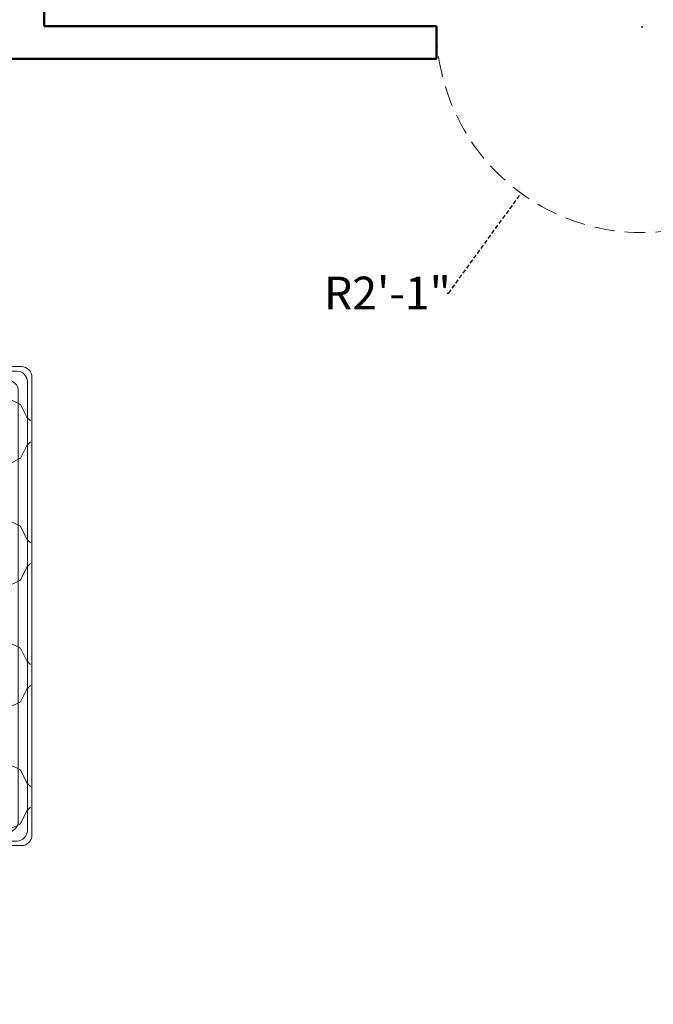
# Model space of a CAD drawing. Units: inches. Extents: x 513 to 1142, y 396 to 927.
# Tile 4 of 31: x 665 to 743, y 522 to 642. Entities that reach past the tile are written whole.
import ezdxf

# ---------------------------------------------------------------- set-up
doc = ezdxf.new("R2010")
doc.units = ezdxf.units.IN
doc.header["$MEASUREMENT"] = 0
doc.linetypes.add('DASHED', pattern=[0.75, 0.5, -0.25])
for name, color, linetype, lineweight in [('A-ANNO-DIMS', 2, 'DASHED', 18), ('A-DOOR-SWNG', 4, 'DASHED', 13), ('A-WALL', 7, 'Continuous', 50), ('furniture', 92, 'Continuous', 18)]:
    doc.layers.add(name, color=color, linetype=linetype, lineweight=lineweight)
doc.styles.get("Standard").update_dxf_attribs({"font": 'arial.ttf'})
doc.dimstyles.get("Standard").update_dxf_attribs({"dimtxt": 4, "dimasz": 0.18, "dimexe": 0.18, "dimexo": 0.0625, "dimgap": 0.09, "dimtad": 0, "dimtih": 1, "dimtoh": 1, "dimdec": 0, "dimrnd": 6, "dimzin": 0, "dimdsep": 46, "dimlunit": 3, "dimtxsty": 'Standard', "dimcen": 0.09, "dimadec": 0, "dimazin": 0, "dimtfac": 1, "dimtdec": 0, "dimtofl": 0, "dimtmove": 0, "dimatfit": 3, "dimfxl": 1, "dimtolj": 1, "dimtzin": 0, "dimarcsym": 0})

# ---------------------------------------------------------------- blocks, each defined once
blk = doc.blocks.new('A$C029D5C69')
for p, q in [((0.4164, 2.0693), (0.4164, 2.0066)), ((2.2315, 2.0693), (0.4164, 2.0693)), ((2.2315, 2.0066), (2.2315, 2.0693)), ((0, 1.606), (0, 2.0066)), ((0, 2.0066), (0.505, 2.0066)), ((0.0151, 1.6211), (0.0151, 1.9915)), ((0.0151, 1.9915), (0.4899, 1.9915)), ((0.4164, 2.0066), (2.2315, 2.0066)), ((0.4899, 1.9915), (0.4899, 1.6211)), ((0.505, 2.0066), (0.505, 1.606)), ((0.5252, 0.0351), (0.5252, 2.0066)), ((0.5403, 0.0502), (0.5403, 2.0066)), ((0.5706, 0.0805), (0.5706, 2.0066)), ((0.6869, 1.966), (0.6666, 2.0066)), ((0.7072, 2.0066), (0.6869, 1.966)), ((1.0902, 1.966), (1.0699, 2.0066)), ((1.1106, 2.0066), (1.0902, 1.966)), ((2.1114, 2.0087), (2.1114, 0.0351)), ((2.6479, 2.0066), (2.1429, 2.0066)), ((2.1429, 2.0066), (2.1429, 1.606)), ((2.6328, 1.9915), (2.158, 1.9915)), ((2.158, 1.9915), (2.158, 1.6211)), ((2.6328, 1.6211), (2.6328, 1.9915)), ((2.6479, 1.606), (2.6479, 2.0066)), ((0.2689, 1.9609), (0.2689, 1.6764)), ((0.6869, 1.9425), (0.6869, 1.966)), ((0.6869, 1.9425), (0.6869, 1.966)), ((1.0902, 1.9425), (1.0902, 1.966)), ((1.0902, 1.9425), (1.0902, 1.966)), ((1.8954, 1.9865), (1.3081, 1.9865)), ((1.8954, 1.9713), (1.3339, 1.9713)), ((1.3849, 1.9713), (1.3656, 1.952)), ((1.3945, 1.9713), (1.3714, 1.9483)), ((1.4249, 1.945), (1.3986, 1.9713)), ((1.4288, 1.9507), (1.4081, 1.9713)), ((1.487, 1.9713), (1.4664, 1.9507)), ((1.4966, 1.9713), (1.4703, 1.945)), ((1.527, 1.945), (1.5007, 1.9713)), ((1.5309, 1.9507), (1.5102, 1.9713)), ((1.5891, 1.9713), (1.5685, 1.9507)), ((1.5987, 1.9713), (1.5724, 1.945)), ((1.6291, 1.945), (1.6028, 1.9713)), ((1.633, 1.9507), (1.6123, 1.9713)), ((1.6912, 1.9713), (1.6706, 1.9507)), ((1.7008, 1.9713), (1.6745, 1.945)), ((1.7312, 1.945), (1.7049, 1.9713)), ((1.7351, 1.9507), (1.7144, 1.9713)), ((1.7933, 1.9713), (1.7727, 1.9507)), ((1.8029, 1.9713), (1.7766, 1.945)), ((1.8333, 1.945), (1.807, 1.9713)), ((1.8372, 1.9507), (1.8165, 1.9713)), ((1.8954, 1.9713), (1.8748, 1.9507)), ((1.9043, 1.9707), (1.8787, 1.945)), ((1.9354, 1.945), (1.9114, 1.969)), ((2.379, 1.9609), (2.379, 1.6764)), ((0.6634, 1.9425), (0.621, 1.9213)), ((0.6634, 1.9425), (0.621, 1.9213)), ((0.6869, 1.9425), (0.6634, 1.9425)), ((0.6869, 1.9425), (0.7104, 1.9425)), ((0.7528, 1.9213), (0.7104, 1.9425)), ((0.7528, 1.9213), (0.7104, 1.9425)), ((1.0668, 1.9425), (1.0244, 1.9213)), ((1.0668, 1.9425), (1.0244, 1.9213)), ((1.0902, 1.9425), (1.0668, 1.9425)), ((1.0902, 1.9425), (1.1137, 1.9425)), ((1.1561, 1.9213), (1.1137, 1.9425)), ((1.1561, 1.9213), (1.1137, 1.9425)), ((1.4249, 1.945), (1.4059, 1.926)), ((1.4288, 1.9394), (1.4116, 1.9222)), ((1.4476, 1.9507), (1.4288, 1.9507)), ((1.4288, 1.9393), (1.4476, 1.9393)), ((1.4476, 1.9507), (1.4664, 1.9507)), ((1.4664, 1.9393), (1.4476, 1.9393)), ((1.493, 1.9128), (1.4664, 1.9394)), ((1.4986, 1.9167), (1.4703, 1.945)), ((1.527, 1.945), (1.4986, 1.9167)), ((1.5309, 1.9394), (1.5043, 1.9128)), ((1.5497, 1.9507), (1.5309, 1.9507)), ((1.5309, 1.9393), (1.5497, 1.9393)), ((1.5497, 1.9507), (1.5685, 1.9507)), ((1.5685, 1.9393), (1.5497, 1.9393)), ((1.595, 1.9128), (1.5685, 1.9394)), ((1.6007, 1.9167), (1.5724, 1.945)), ((1.6291, 1.945), (1.6007, 1.9167)), ((1.633, 1.9394), (1.6064, 1.9128)), ((1.6518, 1.9507), (1.633, 1.9507)), ((1.633, 1.9393), (1.6518, 1.9393)), ((1.6518, 1.9507), (1.6706, 1.9507)), ((1.6706, 1.9393), (1.6518, 1.9393)), ((1.6971, 1.9128), (1.6706, 1.9394)), ((1.7028, 1.9167), (1.6745, 1.945)), ((1.7312, 1.945), (1.7028, 1.9167)), ((1.7351, 1.9394), (1.7085, 1.9128)), ((1.7539, 1.9507), (1.7351, 1.9507)), ((1.7351, 1.9393), (1.7539, 1.9393)), ((1.7539, 1.9507), (1.7727, 1.9507)), ((1.7727, 1.9393), (1.7539, 1.9393)), ((1.7992, 1.9128), (1.7727, 1.9394)), ((1.8049, 1.9167), (1.7766, 1.945)), ((1.8333, 1.945), (1.8049, 1.9167)), ((1.8372, 1.9394), (1.8106, 1.9128)), ((1.856, 1.9507), (1.8372, 1.9507)), ((1.8372, 1.9393), (1.856, 1.9393)), ((1.856, 1.9507), (1.8748, 1.9507)), ((1.8748, 1.9393), (1.856, 1.9393)), ((1.9013, 1.9128), (1.8748, 1.9394)), ((1.907, 1.9167), (1.8787, 1.945)), ((1.9354, 1.945), (1.907, 1.9167)), ((1.9393, 1.9394), (1.9127, 1.9128)), ((1.9393, 1.9393), (1.9404, 1.9393)), ((1.9414, 1.688), (1.9414, 1.931)), ((1.9565, 1.688), (1.9565, 1.931)), ((0.5955, 1.8958), (0.5743, 1.8534)), ((0.621, 1.9213), (0.5955, 1.8958)), ((0.7783, 1.8958), (0.7528, 1.9213)), ((0.7995, 1.8534), (0.7783, 1.8958)), ((0.9989, 1.8958), (0.9777, 1.8534)), ((1.0243, 1.9213), (0.9988, 1.8958)), ((1.1816, 1.8958), (1.1561, 1.9213)), ((1.2028, 1.8534), (1.1816, 1.8958)), ((1.493, 1.8752), (1.493, 1.9128)), ((1.5043, 1.8752), (1.5043, 1.9128)), ((1.595, 1.8752), (1.595, 1.9128)), ((1.6064, 1.8752), (1.6064, 1.9128)), ((1.6971, 1.8752), (1.6971, 1.9128)), ((1.7085, 1.8752), (1.7085, 1.9128)), ((1.7992, 1.8752), (1.7992, 1.9128)), ((1.8106, 1.8752), (1.8106, 1.9128)), ((1.9013, 1.8752), (1.9013, 1.9128)), ((1.9127, 1.8752), (1.9127, 1.9128)), ((1.493, 1.8752), (1.4867, 1.869)), ((1.4986, 1.8713), (1.4922, 1.8648)), ((1.527, 1.8429), (1.4986, 1.8713)), ((1.5309, 1.8486), (1.5043, 1.8752)), ((1.595, 1.8752), (1.5685, 1.8486)), ((1.6007, 1.8713), (1.5724, 1.8429)), ((1.6291, 1.8429), (1.6007, 1.8713)), ((1.633, 1.8486), (1.6064, 1.8752)), ((1.6971, 1.8752), (1.6706, 1.8486)), ((1.7028, 1.8713), (1.6745, 1.8429)), ((1.7312, 1.8429), (1.7028, 1.8713)), ((1.7351, 1.8486), (1.7085, 1.8752)), ((1.7992, 1.8752), (1.7727, 1.8486)), ((1.8049, 1.8713), (1.7766, 1.8429)), ((1.8333, 1.8429), (1.8049, 1.8713)), ((1.8372, 1.8486), (1.8106, 1.8752)), ((1.9013, 1.8752), (1.8748, 1.8486)), ((1.907, 1.8713), (1.8787, 1.8429)), ((1.9354, 1.8429), (1.907, 1.8713)), ((1.9393, 1.8486), (1.9127, 1.8752)), ((0.5743, 1.8534), (0.5706, 1.8515)), ((0.5743, 1.8534), (0.5706, 1.8515)), ((0.8419, 1.8322), (0.7995, 1.8534)), ((0.8419, 1.8322), (0.7995, 1.8534)), ((0.8674, 1.8067), (0.8419, 1.8322)), ((0.9352, 1.8322), (0.9097, 1.8067)), ((0.9777, 1.8534), (0.9353, 1.8322)), ((0.9777, 1.8534), (0.9353, 1.8322)), ((1.2452, 1.8322), (1.2028, 1.8534)), ((1.2452, 1.8322), (1.2028, 1.8534)), ((1.2707, 1.8067), (1.2452, 1.8322)), ((1.527, 1.8429), (1.5242, 1.8401)), ((1.5309, 1.8373), (1.5295, 1.8359)), ((1.5497, 1.8486), (1.5309, 1.8486)), ((1.5309, 1.8373), (1.5497, 1.8373)), ((1.5497, 1.8486), (1.5685, 1.8486)), ((1.5685, 1.8373), (1.5497, 1.8373)), ((1.595, 1.8107), (1.5685, 1.8373)), ((1.6007, 1.8146), (1.5724, 1.8429)), ((1.6291, 1.8429), (1.6007, 1.8146)), ((1.633, 1.8373), (1.6064, 1.8107)), ((1.6518, 1.8486), (1.633, 1.8486)), ((1.633, 1.8373), (1.6518, 1.8373)), ((1.6518, 1.8486), (1.6706, 1.8486)), ((1.6706, 1.8373), (1.6518, 1.8373)), ((1.6971, 1.8107), (1.6706, 1.8373)), ((1.7028, 1.8146), (1.6745, 1.8429)), ((1.7312, 1.8429), (1.7028, 1.8146)), ((1.7351, 1.8373), (1.7085, 1.8107)), ((1.7539, 1.8486), (1.7351, 1.8486)), ((1.7351, 1.8373), (1.7539, 1.8373)), ((1.7539, 1.8486), (1.7727, 1.8486)), ((1.7727, 1.8373), (1.7539, 1.8373)), ((1.7992, 1.8107), (1.7727, 1.8373)), ((1.8049, 1.8146), (1.7766, 1.8429)), ((1.8333, 1.8429), (1.8049, 1.8146)), ((1.8372, 1.8373), (1.8106, 1.8107)), ((1.856, 1.8486), (1.8372, 1.8486)), ((1.8372, 1.8373), (1.856, 1.8373)), ((1.856, 1.8486), (1.8748, 1.8486)), ((1.8748, 1.8373), (1.856, 1.8373)), ((1.9013, 1.8107), (1.8748, 1.8373)), ((1.907, 1.8146), (1.8787, 1.8429)), ((1.9354, 1.8429), (1.907, 1.8146)), ((1.9393, 1.8373), (1.9127, 1.8107)), ((1.9414, 1.8486), (1.9393, 1.8486)), ((1.9393, 1.8373), (1.9414, 1.8373)), ((0.1267, 1.8186), (0.4111, 1.8186)), ((0.8886, 1.7643), (0.8674, 1.8067)), ((0.9098, 1.8067), (0.8886, 1.7643)), ((1.2919, 1.7643), (1.2707, 1.8067)), ((1.595, 1.7806), (1.595, 1.8107)), ((1.6064, 1.7731), (1.6064, 1.8107)), ((1.6971, 1.7731), (1.6971, 1.8107)), ((1.7085, 1.7731), (1.7085, 1.8107)), ((1.7992, 1.7731), (1.7992, 1.8107)), ((1.8106, 1.7731), (1.8106, 1.8107)), ((1.9013, 1.7731), (1.9013, 1.8107)), ((1.9127, 1.7731), (1.9127, 1.8107)), ((2.2367, 1.8186), (2.5212, 1.8186)), ((0.8886, 1.7408), (0.8886, 1.7643)), ((1.2981, 1.7768), (1.2919, 1.7643)), ((1.2919, 1.7519), (1.2919, 1.7643)), ((1.633, 1.7465), (1.6064, 1.7731)), ((1.6971, 1.7731), (1.6706, 1.7465)), ((1.7028, 1.7692), (1.6745, 1.7408)), ((1.7312, 1.7408), (1.7028, 1.7692)), ((1.7351, 1.7465), (1.7085, 1.7731)), ((1.7992, 1.7731), (1.7727, 1.7465)), ((1.8049, 1.7692), (1.7766, 1.7408)), ((1.8333, 1.7408), (1.8049, 1.7692)), ((1.8372, 1.7465), (1.8106, 1.7731)), ((1.9013, 1.7731), (1.8748, 1.7465)), ((1.907, 1.7692), (1.8787, 1.7408)), ((1.9354, 1.7408), (1.907, 1.7692)), ((1.9393, 1.7465), (1.9127, 1.7731)), ((0.8651, 1.7408), (0.8227, 1.7196)), ((0.8651, 1.7408), (0.8227, 1.7196)), ((0.912, 1.7408), (0.8651, 1.7408)), ((0.9544, 1.7196), (0.912, 1.7408)), ((0.9544, 1.7196), (0.912, 1.7408)), ((1.2684, 1.7408), (1.226, 1.7196)), ((1.2684, 1.7408), (1.226, 1.7196)), ((1.2885, 1.7408), (1.2684, 1.7408)), ((1.6518, 1.7465), (1.633, 1.7465)), ((1.6443, 1.7352), (1.6518, 1.7352)), ((1.6518, 1.7465), (1.6706, 1.7465)), ((1.6706, 1.7352), (1.6518, 1.7352)), ((1.6971, 1.7086), (1.6706, 1.7352)), ((1.7028, 1.7125), (1.6745, 1.7408)), ((1.7312, 1.7408), (1.7028, 1.7125)), ((1.7351, 1.7352), (1.7085, 1.7086)), ((1.7539, 1.7465), (1.7351, 1.7465)), ((1.7351, 1.7352), (1.7539, 1.7352)), ((1.7539, 1.7465), (1.7727, 1.7465)), ((1.7727, 1.7352), (1.7539, 1.7352)), ((1.7992, 1.7086), (1.7727, 1.7352)), ((1.8049, 1.7125), (1.7766, 1.7408)), ((1.8333, 1.7408), (1.8049, 1.7125)), ((1.8372, 1.7352), (1.8106, 1.7086)), ((1.856, 1.7465), (1.8372, 1.7465)), ((1.8372, 1.7352), (1.856, 1.7352)), ((1.856, 1.7465), (1.8748, 1.7465)), ((1.8748, 1.7352), (1.856, 1.7352)), ((1.9013, 1.7086), (1.8748, 1.7352)), ((1.907, 1.7125), (1.8787, 1.7408)), ((1.9354, 1.7408), (1.907, 1.7125)), ((1.9393, 1.7352), (1.9127, 1.7086)), ((1.9414, 1.7465), (1.9393, 1.7465)), ((1.9393, 1.7352), (1.9414, 1.7352)), ((0.5766, 1.6941), (0.5706, 1.7002)), ((0.8227, 1.7196), (0.7972, 1.6941)), ((0.98, 1.6941), (0.9545, 1.7196)), ((1.226, 1.7196), (1.2005, 1.6941)), ((1.6971, 1.682), (1.6971, 1.7086)), ((1.7085, 1.671), (1.7085, 1.7086)), ((1.7992, 1.671), (1.7992, 1.7086)), ((1.8106, 1.671), (1.8106, 1.7086)), ((1.9013, 1.671), (1.9013, 1.7086)), ((1.9127, 1.671), (1.9127, 1.7086)), ((2.5551, 1.6275), (2.5551, 1.696)), ((0.5978, 1.6517), (0.5766, 1.6941)), ((0.7972, 1.6941), (0.776, 1.6517)), ((1.0011, 1.6517), (0.9799, 1.6941)), ((1.2005, 1.6941), (1.1793, 1.6517)), ((1.7318, 1.6477), (1.7085, 1.671)), ((1.7992, 1.671), (1.7759, 1.6477)), ((1.8049, 1.6671), (1.7855, 1.6477)), ((1.8244, 1.6477), (1.8049, 1.6671)), ((1.8339, 1.6477), (1.8106, 1.671)), ((1.9013, 1.671), (1.878, 1.6477)), ((1.907, 1.6671), (1.8876, 1.6477)), ((1.9202, 1.6539), (1.907, 1.6671)), ((1.926, 1.6577), (1.9127, 1.671)), ((0.6402, 1.6305), (0.5978, 1.6517)), ((0.6402, 1.6305), (0.5978, 1.6517)), ((0.6657, 1.605), (0.6402, 1.6305)), ((0.7336, 1.6305), (0.7081, 1.605)), ((0.776, 1.6517), (0.7336, 1.6305)), ((0.776, 1.6517), (0.7336, 1.6305)), ((1.0435, 1.6305), (1.0011, 1.6517)), ((1.0435, 1.6305), (1.0011, 1.6517)), ((1.0691, 1.605), (1.0436, 1.6305)), ((1.1369, 1.6305), (1.1114, 1.605)), ((1.1793, 1.6517), (1.1369, 1.6305)), ((1.1793, 1.6517), (1.1369, 1.6305)), ((1.8961, 1.6477), (1.7289, 1.6477)), ((1.8961, 1.6325), (1.7422, 1.6325)), ((0.505, 1.606), (0, 1.606)), ((0.4899, 1.6211), (0.0151, 1.6211)), ((0.6869, 1.5626), (0.6657, 1.605)), ((0.7081, 1.605), (0.6869, 1.5626)), ((1.0902, 1.5626), (1.069, 1.605)), ((1.1114, 1.605), (1.0902, 1.5626)), ((2.1429, 1.606), (2.6479, 1.606)), ((2.158, 1.6211), (2.6328, 1.6211)), ((0.6634, 1.5391), (0.621, 1.5179)), ((0.6634, 1.5391), (0.621, 1.5179)), ((0.6869, 1.5392), (0.6634, 1.5392)), ((0.6869, 1.5392), (0.6869, 1.5626)), ((0.6869, 1.5392), (0.6869, 1.5626)), ((0.6869, 1.5392), (0.7104, 1.5392)), ((0.7528, 1.5179), (0.7104, 1.5391)), ((0.7528, 1.5179), (0.7104, 1.5391)), ((1.0668, 1.5391), (1.0244, 1.5179)), ((1.0668, 1.5391), (1.0244, 1.5179)), ((1.0902, 1.5392), (1.0668, 1.5392)), ((1.0902, 1.5392), (1.0902, 1.5626)), ((1.0902, 1.5392), (1.0902, 1.5626)), ((1.0902, 1.5392), (1.1137, 1.5392)), ((1.1561, 1.5179), (1.1137, 1.5391)), ((1.1561, 1.5179), (1.1137, 1.5391)), ((0.621, 1.5179), (0.5955, 1.4924)), ((0.7783, 1.4924), (0.7528, 1.5179)), ((1.0243, 1.5179), (0.9988, 1.4924)), ((1.1816, 1.4924), (1.1561, 1.5179)), ((1.4277, 1.5179), (1.4022, 1.4924)), ((1.4534, 1.5308), (1.4277, 1.5179)), ((1.4534, 1.5308), (1.4277, 1.5179)), ((0.5955, 1.4925), (0.5743, 1.4501)), ((0.7995, 1.4501), (0.7783, 1.4925)), ((0.9989, 1.4925), (0.9777, 1.4501)), ((1.2028, 1.4501), (1.1816, 1.4925)), ((1.4022, 1.4925), (1.381, 1.4501)), ((1.6062, 1.4501), (1.5966, 1.4692)), ((0.5743, 1.45), (0.5706, 1.4481)), ((0.5743, 1.45), (0.5706, 1.4481)), ((0.8419, 1.4288), (0.7995, 1.45)), ((0.8419, 1.4288), (0.7995, 1.45)), ((0.9777, 1.45), (0.9353, 1.4288)), ((0.9777, 1.45), (0.9353, 1.4288)), ((1.2452, 1.4288), (1.2028, 1.45)), ((1.2452, 1.4288), (1.2028, 1.45)), ((1.381, 1.45), (1.3386, 1.4288)), ((1.381, 1.45), (1.3386, 1.4288)), ((1.6486, 1.4288), (1.6062, 1.45)), ((1.6486, 1.4288), (1.6062, 1.45)), ((0.5403, 1.4117), (0.5706, 1.4117)), ((0.8674, 1.4033), (0.8419, 1.4288)), ((0.8886, 1.361), (0.8674, 1.4034)), ((0.9098, 1.4034), (0.8886, 1.361)), ((0.9352, 1.4288), (0.9097, 1.4033)), ((1.2707, 1.4033), (1.2452, 1.4288)), ((1.2919, 1.361), (1.2707, 1.4034)), ((1.3131, 1.4034), (1.2919, 1.361)), ((1.3386, 1.4288), (1.3131, 1.4033)), ((1.6741, 1.4033), (1.6486, 1.4288)), ((1.6953, 1.361), (1.6741, 1.4034)), ((1.714, 1.3984), (1.6953, 1.361)), ((0.8651, 1.3374), (0.8227, 1.3162)), ((0.8651, 1.3374), (0.8227, 1.3162)), ((0.912, 1.3375), (0.8651, 1.3375)), ((0.8886, 1.3375), (0.8886, 1.3609)), ((0.9544, 1.3162), (0.912, 1.3374)), ((0.9544, 1.3162), (0.912, 1.3374)), ((1.2684, 1.3374), (1.226, 1.3162)), ((1.2684, 1.3374), (1.226, 1.3162)), ((1.3154, 1.3375), (1.2684, 1.3375)), ((1.2919, 1.3375), (1.2919, 1.3609)), ((1.3578, 1.3162), (1.3154, 1.3374)), ((1.3578, 1.3162), (1.3154, 1.3374)), ((1.6718, 1.3374), (1.6294, 1.3162)), ((1.6718, 1.3374), (1.6294, 1.3162)), ((1.7187, 1.3375), (1.6718, 1.3375)), ((1.6953, 1.3375), (1.6953, 1.3609)), ((1.7611, 1.3162), (1.7187, 1.3374)), ((1.7611, 1.3162), (1.7187, 1.3374)), ((0.8227, 1.3163), (0.7972, 1.2908)), ((0.98, 1.2908), (0.9545, 1.3163)), ((1.226, 1.3163), (1.2005, 1.2908)), ((1.3833, 1.2908), (1.3578, 1.3163)), ((1.6294, 1.3163), (1.6039, 1.2908)), ((1.7867, 1.2908), (1.7611, 1.3163)), ((0.5766, 1.2908), (0.5706, 1.2968)), ((0.5978, 1.2484), (0.5766, 1.2908)), ((0.7972, 1.2908), (0.776, 1.2484)), ((1.0011, 1.2484), (0.9799, 1.2908)), ((1.2005, 1.2908), (1.1793, 1.2484)), ((1.4045, 1.2484), (1.3833, 1.2908)), ((1.6039, 1.2908), (1.5827, 1.2484)), ((1.8078, 1.2484), (1.7866, 1.2908)), ((0.6402, 1.2271), (0.5978, 1.2483)), ((0.6402, 1.2271), (0.5978, 1.2483)), ((0.776, 1.2483), (0.7336, 1.2271)), ((0.776, 1.2483), (0.7336, 1.2271)), ((1.0435, 1.2271), (1.0011, 1.2483)), ((1.0435, 1.2271), (1.0011, 1.2483)), ((1.1793, 1.2483), (1.1369, 1.2271)), ((1.1793, 1.2483), (1.1369, 1.2271)), ((1.4469, 1.2271), (1.4045, 1.2483)), ((1.4469, 1.2271), (1.4045, 1.2483)), ((1.5827, 1.2483), (1.5403, 1.2271)), ((1.5827, 1.2483), (1.5403, 1.2271)), ((1.8502, 1.2271), (1.8078, 1.2483)), ((1.8502, 1.2271), (1.8078, 1.2483)), ((0.5403, 1.21), (0.5706, 1.21)), ((0.6657, 1.2017), (0.6402, 1.2272)), ((0.7336, 1.2272), (0.7081, 1.2017)), ((1.0691, 1.2017), (1.0436, 1.2272)), ((1.1369, 1.2272), (1.1114, 1.2017)), ((1.4724, 1.2017), (1.4469, 1.2272)), ((1.5403, 1.2272), (1.5148, 1.2017)), ((1.8758, 1.2017), (1.8503, 1.2272)), ((0.6869, 1.1593), (0.6657, 1.2017)), ((0.7081, 1.2017), (0.6869, 1.1593)), ((1.0902, 1.1593), (1.069, 1.2017)), ((1.1114, 1.2017), (1.0902, 1.1593)), ((1.4936, 1.1593), (1.4724, 1.2017)), ((1.5148, 1.2017), (1.4936, 1.1593)), ((1.8969, 1.1593), (1.8757, 1.2017)), ((1.9181, 1.2017), (1.8969, 1.1593)), ((1.9215, 1.2051), (1.9181, 1.2017)), ((0.6869, 1.1358), (0.6869, 1.1593)), ((0.6869, 1.1358), (0.6869, 1.1593)), ((1.0902, 1.1358), (1.0902, 1.1593)), ((1.0902, 1.1358), (1.0902, 1.1593)), ((1.4936, 1.1358), (1.4936, 1.1593)), ((1.4936, 1.1358), (1.4936, 1.1593)), ((1.8969, 1.1358), (1.8969, 1.1593)), ((1.8969, 1.1358), (1.8969, 1.1593)), ((0.621, 1.1146), (0.5955, 1.0891)), ((0.6634, 1.1358), (0.621, 1.1146)), ((0.6634, 1.1358), (0.621, 1.1146)), ((0.6869, 1.1358), (0.6634, 1.1358)), ((0.6869, 1.1358), (0.7104, 1.1358)), ((0.7528, 1.1146), (0.7104, 1.1358)), ((0.7528, 1.1146), (0.7104, 1.1358)), ((0.7783, 1.0891), (0.7528, 1.1146)), ((1.0243, 1.1146), (0.9988, 1.0891)), ((1.0668, 1.1358), (1.0244, 1.1146)), ((1.0668, 1.1358), (1.0244, 1.1146)), ((1.0902, 1.1358), (1.0668, 1.1358)), ((1.0902, 1.1358), (1.1137, 1.1358)), ((1.1561, 1.1146), (1.1137, 1.1358)), ((1.1561, 1.1146), (1.1137, 1.1358)), ((1.1816, 1.0891), (1.1561, 1.1146)), ((1.4277, 1.1146), (1.4022, 1.0891)), ((1.4701, 1.1358), (1.4277, 1.1146)), ((1.4701, 1.1358), (1.4277, 1.1146)), ((1.4936, 1.1358), (1.4701, 1.1358)), ((1.4936, 1.1358), (1.5171, 1.1358)), ((1.5595, 1.1146), (1.5171, 1.1358)), ((1.5595, 1.1146), (1.5171, 1.1358)), ((1.585, 1.0891), (1.5595, 1.1146)), ((1.831, 1.1146), (1.8055, 1.0891)), ((1.8735, 1.1358), (1.8311, 1.1146)), ((1.8735, 1.1358), (1.8311, 1.1146)), ((1.8969, 1.1358), (1.8735, 1.1358)), ((1.8969, 1.1358), (1.9204, 1.1358)), ((1.9628, 1.1146), (1.9204, 1.1358)), ((1.9628, 1.1146), (1.9204, 1.1358)), ((1.9883, 1.0891), (1.9628, 1.1146)), ((0.5955, 1.0891), (0.5743, 1.0467)), ((0.7995, 1.0467), (0.7783, 1.0891)), ((0.9989, 1.0891), (0.9777, 1.0467)), ((1.2028, 1.0467), (1.1816, 1.0891)), ((1.4022, 1.0891), (1.381, 1.0467)), ((1.6062, 1.0467), (1.585, 1.0891)), ((1.8056, 1.0891), (1.7844, 1.0467)), ((2.0095, 1.0467), (1.9883, 1.0891)), ((0.5743, 1.0467), (0.5706, 1.0448)), ((0.5743, 1.0467), (0.5706, 1.0448)), ((0.8419, 1.0255), (0.7995, 1.0467)), ((0.8419, 1.0255), (0.7995, 1.0467)), ((0.9777, 1.0467), (0.9353, 1.0255)), ((0.9777, 1.0467), (0.9353, 1.0255)), ((1.2452, 1.0255), (1.2028, 1.0467)), ((1.2452, 1.0255), (1.2028, 1.0467)), ((1.381, 1.0467), (1.3386, 1.0255)), ((1.381, 1.0467), (1.3386, 1.0255)), ((1.6486, 1.0255), (1.6062, 1.0467)), ((1.6486, 1.0255), (1.6062, 1.0467)), ((1.7844, 1.0467), (1.742, 1.0255)), ((1.7844, 1.0467), (1.742, 1.0255)), ((2.0276, 1.0376), (2.0095, 1.0467)), ((2.0276, 1.0376), (2.0095, 1.0467)), ((0.8674, 1), (0.8419, 1.0255)), ((0.9352, 1.0255), (0.9097, 1)), ((1.2707, 1), (1.2452, 1.0255)), ((1.3386, 1.0255), (1.3131, 1)), ((1.6741, 1), (1.6486, 1.0255)), ((1.7419, 1.0255), (1.7164, 1)), ((0.8886, 0.9576), (0.8674, 1)), ((0.9098, 1), (0.8886, 0.9576)), ((1.2919, 0.9576), (1.2707, 1)), ((1.3131, 1), (1.2919, 0.9576)), ((1.6953, 0.9576), (1.6741, 1)), ((1.7165, 1), (1.6953, 0.9576)), ((0.8886, 0.9341), (0.8886, 0.9576)), ((1.2919, 0.9341), (1.2919, 0.9576)), ((1.6953, 0.9341), (1.6953, 0.9576)), ((2.066, 0.9457), (2.066, 0.0805)), ((0.8227, 0.9129), (0.7972, 0.8874)), ((0.8651, 0.9341), (0.8227, 0.9129)), ((0.8651, 0.9341), (0.8227, 0.9129)), ((0.912, 0.9341), (0.8651, 0.9341)), ((0.9544, 0.9129), (0.912, 0.9341)), ((0.9544, 0.9129), (0.912, 0.9341)), ((0.98, 0.8874), (0.9545, 0.9129)), ((1.226, 0.9129), (1.2005, 0.8874)), ((1.2684, 0.9341), (1.226, 0.9129)), ((1.2684, 0.9341), (1.226, 0.9129)), ((1.3154, 0.9341), (1.2684, 0.9341)), ((1.3578, 0.9129), (1.3154, 0.9341)), ((1.3578, 0.9129), (1.3154, 0.9341)), ((1.3833, 0.8874), (1.3578, 0.9129)), ((1.6294, 0.9129), (1.6039, 0.8874)), ((1.6718, 0.9341), (1.6294, 0.9129)), ((1.6718, 0.9341), (1.6294, 0.9129)), ((1.7187, 0.9341), (1.6718, 0.9341)), ((1.7611, 0.9129), (1.7187, 0.9341)), ((1.7611, 0.9129), (1.7187, 0.9341)), ((1.7867, 0.8874), (1.7611, 0.9129)), ((2.0327, 0.9129), (2.0072, 0.8874)), ((2.066, 0.9295), (2.0327, 0.9129)), ((2.066, 0.9295), (2.0327, 0.9129)), ((0.5766, 0.8874), (0.5706, 0.8935)), ((0.5978, 0.845), (0.5766, 0.8874)), ((0.7972, 0.8874), (0.776, 0.845)), ((1.0011, 0.845), (0.9799, 0.8874)), ((1.2005, 0.8874), (1.1793, 0.845)), ((1.4045, 0.845), (1.3833, 0.8874)), ((1.6039, 0.8874), (1.5827, 0.845)), ((1.8078, 0.845), (1.7866, 0.8874)), ((2.0072, 0.8874), (1.986, 0.845)), ((0.6402, 0.8238), (0.5978, 0.845)), ((0.6402, 0.8238), (0.5978, 0.845)), ((0.6657, 0.7983), (0.6402, 0.8238)), ((0.7336, 0.8238), (0.7081, 0.7983)), ((0.776, 0.845), (0.7336, 0.8238)), ((0.776, 0.845), (0.7336, 0.8238)), ((1.0435, 0.8238), (1.0011, 0.845)), ((1.0435, 0.8238), (1.0011, 0.845)), ((1.0691, 0.7983), (1.0436, 0.8238)), ((1.1369, 0.8238), (1.1114, 0.7983)), ((1.1793, 0.845), (1.1369, 0.8238)), ((1.1793, 0.845), (1.1369, 0.8238)), ((1.4469, 0.8238), (1.4045, 0.845)), ((1.4469, 0.8238), (1.4045, 0.845)), ((1.4724, 0.7983), (1.4469, 0.8238)), ((1.5403, 0.8238), (1.5148, 0.7983)), ((1.5827, 0.845), (1.5403, 0.8238)), ((1.5827, 0.845), (1.5403, 0.8238)), ((1.8502, 0.8238), (1.8078, 0.845)), ((1.8502, 0.8238), (1.8078, 0.845)), ((1.8758, 0.7983), (1.8503, 0.8238)), ((1.9436, 0.8238), (1.9181, 0.7983)), ((1.986, 0.845), (1.9436, 0.8238)), ((1.986, 0.845), (1.9436, 0.8238)), ((2.0962, 0.8369), (2.0962, 0.0502)), ((0.6869, 0.7559), (0.6657, 0.7983)), ((0.7081, 0.7983), (0.6869, 0.7559)), ((1.0902, 0.7559), (1.069, 0.7983)), ((1.1114, 0.7983), (1.0902, 0.7559)), ((1.4936, 0.7559), (1.4724, 0.7983)), ((1.5148, 0.7983), (1.4936, 0.7559)), ((1.8969, 0.7559), (1.8757, 0.7983)), ((1.9181, 0.7983), (1.8969, 0.7559)), ((0.6869, 0.7325), (0.6869, 0.7559)), ((0.6869, 0.7325), (0.6869, 0.7559)), ((1.0902, 0.7325), (1.0902, 0.7559)), ((1.0902, 0.7325), (1.0902, 0.7559)), ((1.2024, 0.7028), (1.2503, 0.7507)), ((1.4936, 0.7325), (1.4936, 0.7559)), ((1.4936, 0.7325), (1.4936, 0.7559)), ((1.8969, 0.7325), (1.8969, 0.7559)), ((1.8969, 0.7325), (1.8969, 0.7559)), ((0.6634, 0.7324), (0.621, 0.7112)), ((0.6634, 0.7324), (0.621, 0.7112)), ((0.6869, 0.7325), (0.6634, 0.7325)), ((0.6869, 0.7325), (0.7104, 0.7325)), ((0.7528, 0.7112), (0.7104, 0.7324)), ((0.7528, 0.7112), (0.7104, 0.7324)), ((1.0668, 0.7324), (1.0244, 0.7112)), ((1.0668, 0.7324), (1.0244, 0.7112)), ((1.0902, 0.7325), (1.0668, 0.7325)), ((1.0902, 0.7325), (1.1137, 0.7325)), ((1.1561, 0.7112), (1.1137, 0.7324)), ((1.1561, 0.7112), (1.1137, 0.7324)), ((1.4701, 0.7324), (1.4277, 0.7112)), ((1.4701, 0.7324), (1.4277, 0.7112)), ((1.4936, 0.7325), (1.4701, 0.7325)), ((1.4936, 0.7325), (1.5171, 0.7325)), ((1.5595, 0.7112), (1.5171, 0.7324)), ((1.5595, 0.7112), (1.5171, 0.7324)), ((1.8735, 0.7324), (1.8311, 0.7112)), ((1.8735, 0.7324), (1.8311, 0.7112)), ((1.8969, 0.7325), (1.8735, 0.7325)), ((1.8969, 0.7325), (1.9204, 0.7325)), ((1.9628, 0.7112), (1.9204, 0.7324)), ((1.9628, 0.7112), (1.9204, 0.7324)), ((0.5955, 0.6858), (0.5743, 0.6434)), ((0.621, 0.7113), (0.5955, 0.6858)), ((0.7783, 0.6858), (0.7528, 0.7113)), ((0.7995, 0.6434), (0.7783, 0.6858)), ((0.9989, 0.6858), (0.9777, 0.6434)), ((1.0243, 0.7113), (0.9988, 0.6858)), ((1.1816, 0.6858), (1.1561, 0.7113)), ((1.2028, 0.6434), (1.1816, 0.6858)), ((1.4022, 0.6858), (1.381, 0.6434)), ((1.4277, 0.7113), (1.4022, 0.6858)), ((1.585, 0.6858), (1.5595, 0.7113)), ((1.6062, 0.6434), (1.585, 0.6858)), ((1.8056, 0.6858), (1.7844, 0.6434)), ((1.831, 0.7113), (1.8055, 0.6858)), ((1.9883, 0.6858), (1.9628, 0.7113)), ((2.0095, 0.6434), (1.9883, 0.6858)), ((0.5743, 0.6433), (0.5706, 0.6414)), ((0.5743, 0.6433), (0.5706, 0.6414)), ((0.8419, 0.6221), (0.7995, 0.6433)), ((0.8419, 0.6221), (0.7995, 0.6433)), ((0.8674, 0.5967), (0.8419, 0.6222)), ((0.9352, 0.6222), (0.9097, 0.5967)), ((0.9777, 0.6433), (0.9353, 0.6221)), ((0.9777, 0.6433), (0.9353, 0.6221)), ((1.2452, 0.6221), (1.2028, 0.6433)), ((1.2452, 0.6221), (1.2028, 0.6433)), ((1.2707, 0.5967), (1.2452, 0.6222)), ((1.3386, 0.6222), (1.3131, 0.5967)), ((1.381, 0.6433), (1.3386, 0.6221)), ((1.381, 0.6433), (1.3386, 0.6221)), ((1.6486, 0.6221), (1.6062, 0.6433)), ((1.6486, 0.6221), (1.6062, 0.6433)), ((1.6741, 0.5967), (1.6486, 0.6222)), ((1.7419, 0.6222), (1.7164, 0.5967)), ((1.7844, 0.6433), (1.742, 0.6221)), ((1.7844, 0.6433), (1.742, 0.6221)), ((2.0519, 0.6221), (2.0095, 0.6433)), ((2.0519, 0.6221), (2.0095, 0.6433)), ((2.066, 0.6081), (2.0519, 0.6222)), ((0.8886, 0.5543), (0.8674, 0.5967)), ((0.9098, 0.5967), (0.8886, 0.5543)), ((1.2919, 0.5543), (1.2707, 0.5967)), ((1.3131, 0.5967), (1.2919, 0.5543)), ((1.6953, 0.5543), (1.6741, 0.5967)), ((1.7165, 0.5967), (1.6953, 0.5543)), ((0.8886, 0.5308), (0.8886, 0.5543)), ((1.2919, 0.5308), (1.2919, 0.5543)), ((1.6953, 0.5308), (1.6953, 0.5543)), ((0.8651, 0.5308), (0.8227, 0.5096)), ((0.8651, 0.5308), (0.8227, 0.5096)), ((0.912, 0.5308), (0.8651, 0.5308)), ((0.9544, 0.5096), (0.912, 0.5308)), ((0.9544, 0.5096), (0.912, 0.5308)), ((1.2684, 0.5308), (1.226, 0.5096)), ((1.2684, 0.5308), (1.226, 0.5096)), ((1.3154, 0.5308), (1.2684, 0.5308)), ((1.3578, 0.5096), (1.3154, 0.5308)), ((1.3578, 0.5096), (1.3154, 0.5308)), ((1.6718, 0.5308), (1.6294, 0.5096)), ((1.6718, 0.5308), (1.6294, 0.5096)), ((1.7187, 0.5308), (1.6718, 0.5308)), ((1.7611, 0.5096), (1.7187, 0.5308)), ((1.7611, 0.5096), (1.7187, 0.5308)), ((2.066, 0.5262), (2.0327, 0.5096)), ((2.066, 0.5262), (2.0327, 0.5096)), ((0.5766, 0.4841), (0.5706, 0.4901)), ((0.8227, 0.5096), (0.7972, 0.4841)), ((0.98, 0.4841), (0.9545, 0.5096)), ((1.226, 0.5096), (1.2005, 0.4841)), ((1.3833, 0.4841), (1.3578, 0.5096)), ((1.6294, 0.5096), (1.6039, 0.4841)), ((1.7867, 0.4841), (1.7611, 0.5096)), ((2.0327, 0.5096), (2.0072, 0.4841)), ((0.5978, 0.4417), (0.5766, 0.4841)), ((0.7972, 0.4841), (0.776, 0.4417)), ((1.0011, 0.4417), (0.9799, 0.4841)), ((1.2005, 0.4841), (1.1793, 0.4417)), ((1.4045, 0.4417), (1.3833, 0.4841)), ((1.6039, 0.4841), (1.5827, 0.4417)), ((1.8078, 0.4417), (1.7866, 0.4841)), ((2.0072, 0.4841), (1.986, 0.4417)), ((0.6402, 0.4205), (0.5978, 0.4417)), ((0.6402, 0.4205), (0.5978, 0.4417)), ((0.776, 0.4417), (0.7336, 0.4205)), ((0.776, 0.4417), (0.7336, 0.4205)), ((1.0435, 0.4205), (1.0011, 0.4417)), ((1.0435, 0.4205), (1.0011, 0.4417)), ((1.1793, 0.4417), (1.1369, 0.4205)), ((1.1793, 0.4417), (1.1369, 0.4205)), ((1.4469, 0.4205), (1.4045, 0.4417)), ((1.4469, 0.4205), (1.4045, 0.4417)), ((1.5827, 0.4417), (1.5403, 0.4205)), ((1.5827, 0.4417), (1.5403, 0.4205)), ((1.8502, 0.4205), (1.8078, 0.4417)), ((1.8502, 0.4205), (1.8078, 0.4417)), ((1.986, 0.4417), (1.9436, 0.4205)), ((1.986, 0.4417), (1.9436, 0.4205)), ((0.6657, 0.395), (0.6402, 0.4205)), ((0.6869, 0.3526), (0.6657, 0.395)), ((0.7081, 0.395), (0.6869, 0.3526)), ((0.7336, 0.4205), (0.7081, 0.395)), ((1.0691, 0.395), (1.0436, 0.4205)), ((1.0902, 0.3526), (1.069, 0.395)), ((1.1114, 0.395), (1.0902, 0.3526)), ((1.1369, 0.4205), (1.1114, 0.395)), ((1.4724, 0.395), (1.4469, 0.4205)), ((1.4936, 0.3526), (1.4724, 0.395)), ((1.5148, 0.395), (1.4936, 0.3526)), ((1.5403, 0.4205), (1.5148, 0.395)), ((1.8758, 0.395), (1.8503, 0.4205)), ((1.8969, 0.3526), (1.8757, 0.395)), ((1.9181, 0.395), (1.8969, 0.3526)), ((1.9436, 0.4205), (1.9181, 0.395)), ((0.6634, 0.3291), (0.621, 0.3079)), ((0.6634, 0.3291), (0.621, 0.3079)), ((0.6869, 0.3291), (0.6634, 0.3291)), ((0.6869, 0.3291), (0.6869, 0.3526)), ((0.6869, 0.3291), (0.6869, 0.3526)), ((0.6869, 0.3291), (0.7104, 0.3291)), ((0.7528, 0.3079), (0.7104, 0.3291)), ((0.7528, 0.3079), (0.7104, 0.3291)), ((1.0668, 0.3291), (1.0244, 0.3079)), ((1.0668, 0.3291), (1.0244, 0.3079)), ((1.0902, 0.3291), (1.0668, 0.3291)), ((1.0902, 0.3291), (1.0902, 0.3526)), ((1.0902, 0.3291), (1.0902, 0.3526)), ((1.0902, 0.3291), (1.1137, 0.3291)), ((1.1561, 0.3079), (1.1137, 0.3291)), ((1.1561, 0.3079), (1.1137, 0.3291)), ((1.4701, 0.3291), (1.4277, 0.3079)), ((1.4701, 0.3291), (1.4277, 0.3079)), ((1.4936, 0.3291), (1.4701, 0.3291)), ((1.4936, 0.3291), (1.4936, 0.3526)), ((1.4936, 0.3291), (1.4936, 0.3526)), ((1.4936, 0.3291), (1.5171, 0.3291)), ((1.5595, 0.3079), (1.5171, 0.3291)), ((1.5595, 0.3079), (1.5171, 0.3291)), ((1.8735, 0.3291), (1.8311, 0.3079)), ((1.8735, 0.3291), (1.8311, 0.3079)), ((1.8969, 0.3291), (1.8735, 0.3291)), ((1.8969, 0.3291), (1.8969, 0.3526)), ((1.8969, 0.3291), (1.8969, 0.3526)), ((1.8969, 0.3291), (1.9204, 0.3291)), ((1.9628, 0.3079), (1.9204, 0.3291)), ((1.9628, 0.3079), (1.9204, 0.3291)), ((0.621, 0.3079), (0.5955, 0.2824)), ((0.7783, 0.2824), (0.7528, 0.3079)), ((1.0243, 0.3079), (0.9988, 0.2824)), ((1.1816, 0.2824), (1.1561, 0.3079)), ((1.4277, 0.3079), (1.4022, 0.2824)), ((1.585, 0.2824), (1.5595, 0.3079)), ((1.831, 0.3079), (1.8055, 0.2824)), ((1.9883, 0.2824), (1.9628, 0.3079)), ((0.5955, 0.2824), (0.5743, 0.24)), ((0.7995, 0.24), (0.7783, 0.2824)), ((0.9989, 0.2824), (0.9777, 0.24)), ((1.2028, 0.24), (1.1816, 0.2824)), ((1.4022, 0.2824), (1.381, 0.24)), ((1.6062, 0.24), (1.585, 0.2824)), ((1.8056, 0.2824), (1.7844, 0.24)), ((2.0095, 0.24), (1.9883, 0.2824)), ((0.5743, 0.24), (0.5706, 0.2381)), ((0.5743, 0.24), (0.5706, 0.2381)), ((0.8419, 0.2188), (0.7995, 0.24)), ((0.8419, 0.2188), (0.7995, 0.24)), ((0.9777, 0.24), (0.9353, 0.2188)), ((0.9777, 0.24), (0.9353, 0.2188)), ((1.2452, 0.2188), (1.2028, 0.24)), ((1.2452, 0.2188), (1.2028, 0.24)), ((1.381, 0.24), (1.3386, 0.2188)), ((1.381, 0.24), (1.3386, 0.2188)), ((1.6486, 0.2188), (1.6062, 0.24)), ((1.6486, 0.2188), (1.6062, 0.24)), ((1.7844, 0.24), (1.742, 0.2188)), ((1.7844, 0.24), (1.742, 0.2188)), ((2.0519, 0.2188), (2.0095, 0.24)), ((2.0519, 0.2188), (2.0095, 0.24)), ((0.8674, 0.1933), (0.8419, 0.2188)), ((0.9352, 0.2188), (0.9097, 0.1933)), ((1.2707, 0.1933), (1.2452, 0.2188)), ((1.3386, 0.2188), (1.3131, 0.1933)), ((1.6741, 0.1933), (1.6486, 0.2188)), ((1.7419, 0.2188), (1.7164, 0.1933)), ((2.066, 0.2047), (2.0519, 0.2188)), ((0.8886, 0.1509), (0.8674, 0.1933)), ((0.9098, 0.1933), (0.8886, 0.1509)), ((1.2919, 0.1509), (1.2707, 0.1933)), ((1.3131, 0.1933), (1.2919, 0.1509)), ((1.6953, 0.1509), (1.6741, 0.1933)), ((1.7165, 0.1933), (1.6953, 0.1509)), ((0.8886, 0.1275), (0.8886, 0.1509)), ((1.2919, 0.1275), (1.2919, 0.1509)), ((1.6953, 0.1275), (1.6953, 0.1509)), ((0.8227, 0.1062), (0.7972, 0.0807)), ((0.8651, 0.1274), (0.8227, 0.1062)), ((0.8651, 0.1274), (0.8227, 0.1062)), ((0.912, 0.1275), (0.8651, 0.1275)), ((0.9544, 0.1062), (0.912, 0.1274)), ((0.9544, 0.1062), (0.912, 0.1274)), ((0.98, 0.0807), (0.9545, 0.1062)), ((1.226, 0.1062), (1.2005, 0.0807)), ((1.2684, 0.1274), (1.226, 0.1062)), ((1.2684, 0.1274), (1.226, 0.1062)), ((1.3154, 0.1275), (1.2684, 0.1275)), ((1.3578, 0.1062), (1.3154, 0.1274)), ((1.3578, 0.1062), (1.3154, 0.1274)), ((1.3833, 0.0807), (1.3578, 0.1062)), ((1.6294, 0.1062), (1.6039, 0.0807)), ((1.6718, 0.1274), (1.6294, 0.1062)), ((1.6718, 0.1274), (1.6294, 0.1062)), ((1.7187, 0.1275), (1.6718, 0.1275)), ((1.7611, 0.1062), (1.7187, 0.1274)), ((1.7611, 0.1062), (1.7187, 0.1274)), ((1.7867, 0.0807), (1.7611, 0.1062)), ((2.0327, 0.1062), (2.0072, 0.0807)), ((2.066, 0.1228), (2.0327, 0.1062)), ((2.066, 0.1228), (2.0327, 0.1062)), ((0.5766, 0.0807), (0.5706, 0.0868)), ((0.5978, 0.0384), (0.5766, 0.0808)), ((0.7972, 0.0808), (0.776, 0.0384)), ((1.0011, 0.0384), (0.9799, 0.0808)), ((1.2005, 0.0808), (1.1793, 0.0384)), ((1.4045, 0.0384), (1.3833, 0.0808)), ((1.6039, 0.0808), (1.5827, 0.0384)), ((1.8078, 0.0384), (1.7866, 0.0808)), ((2.0072, 0.0808), (1.986, 0.0384)), ((0.6402, 0.0171), (0.5978, 0.0383)), ((0.6402, 0.0171), (0.5978, 0.0383)), ((2.0309, 0.0454), (0.6056, 0.0454)), ((0.776, 0.0383), (0.7336, 0.0171)), ((0.776, 0.0383), (0.7336, 0.0171)), ((1.0435, 0.0171), (1.0011, 0.0383)), ((1.0435, 0.0171), (1.0011, 0.0383)), ((1.1793, 0.0383), (1.1369, 0.0171)), ((1.1793, 0.0383), (1.1369, 0.0171)), ((1.4469, 0.0171), (1.4045, 0.0383)), ((1.4469, 0.0171), (1.4045, 0.0383)), ((1.5827, 0.0383), (1.5403, 0.0171)), ((1.5827, 0.0383), (1.5403, 0.0171)), ((1.8502, 0.0171), (1.8078, 0.0383)), ((1.8502, 0.0171), (1.8078, 0.0383)), ((1.986, 0.0383), (1.9436, 0.0171)), ((1.986, 0.0383), (1.9436, 0.0171)), ((2.0763, 0), (0.5603, 0)), ((2.0612, 0.0151), (0.5754, 0.0151)), ((0.6523, 0.005), (0.6402, 0.0171)), ((0.7336, 0.0171), (0.7215, 0.005)), ((1.0557, 0.005), (1.0436, 0.0171)), ((1.1369, 0.0171), (1.1248, 0.005)), ((1.459, 0.005), (1.4469, 0.0171)), ((1.5403, 0.0171), (1.5282, 0.005)), ((1.8623, 0.005), (1.8503, 0.0171)), ((1.9436, 0.0171), (1.9315, 0.005))]:
    blk.add_line(p, q)
at = {"ltscale": 0.005}
for p, q in [((0.4899, 1.6568), (0.0151, 1.9915)), ((0.0151, 1.6568), (0.4899, 1.9915)), ((2.6328, 1.6568), (2.158, 1.9915)), ((2.158, 1.6568), (2.6328, 1.9915)), ((0.0151, 1.6568), (0.4899, 1.6568)), ((2.6328, 1.6568), (2.158, 1.6568))]:
    blk.add_line(p, q, dxfattribs=at)
for centre, radius in [((0.2689, 1.8186), 0.1191), ((2.379, 1.8186), 0.1191), ((0.2689, 1.8186), 0.0711), ((2.379, 1.8186), 0.0711)]:
    blk.add_circle(centre, radius)
for centre, radius, start, end in [((0.2843, 0.0157), 0.6251, 10.2961, 13.2684), ((0.6056, 0.0805), 0.0351, 180, 270), ((2.0309, 0.0805), 0.0351, 270, 0), ((0.5603, 0.0351), 0.0351, 180, 270), ((0.5754, 0.0502), 0.0351, 180, 270), ((2.0612, 0.0502), 0.0351, 270, 0), ((2.0763, 0.0351), 0.0351, 270, 0)]:
    blk.add_arc(centre, radius, start, end)
for centre, major_axis, ratio, start_param, end_param in [((0.8506, 1.8527), (-0.4556, 0), 0.89, 2.430919, 3.53111), ((0.3667, 0.6698), (1.7398, 0.1668), 0.88072, -0.045073, 0.941433), ((1.8961, 1.931), (-0.0453, 0), 0.89, 3.141593, 4.712389), ((1.8961, 1.688), (-0.0453, 0), 0.89, 1.570796, 3.141593), ((1.0874, 0.6748), (1.021, 0.1213), 0.889348, -0.031673, 1.359628)]:
    blk.add_ellipse(centre, major_axis=major_axis, ratio=ratio, start_param=start_param, end_param=end_param)
for points, knots in [([(1.9565, 1.931), (1.9565, 1.9336), (1.9563, 1.9362), (1.9553, 1.9428), (1.9543, 1.9467), (1.9512, 1.9541), (1.9493, 1.9577), (1.9446, 1.9643), (1.942, 1.9674), (1.936, 1.9729), (1.9327, 1.9753), (1.9257, 1.9795), (1.922, 1.9813), (1.9142, 1.9841), (1.9102, 1.9851), (1.9028, 1.9862), (1.8995, 1.9865), (1.8961, 1.9865)], [3.141593, 3.141593, 3.141593, 3.141593, 3.277614, 3.277614, 3.488082, 3.488082, 3.698551, 3.698551, 3.909019, 3.909019, 4.119488, 4.119488, 4.329956, 4.329956, 4.540424, 4.540424, 4.712389, 4.712389, 4.712389, 4.712389]), ([(1.8961, 1.6325), (1.899, 1.6325), (1.9019, 1.6327), (1.9101, 1.6338), (1.9153, 1.6352), (1.9253, 1.6392), (1.93, 1.6418), (1.9385, 1.6481), (1.9423, 1.6519), (1.9481, 1.6594), (1.9503, 1.663), (1.9537, 1.6707), (1.955, 1.6747), (1.9563, 1.6818), (1.9565, 1.6849), (1.9565, 1.688)], [1.570796, 1.570796, 1.570796, 1.570796, 1.718836, 1.718836, 1.993452, 1.993452, 2.268068, 2.268068, 2.542684, 2.542684, 2.761386, 2.761386, 2.980087, 2.980087, 3.141593, 3.141593, 3.141593, 3.141593])]:
    blk.add_open_spline(points, degree=3, knots=knots)
blk = doc.blocks.new('A$C0D3A6DFA')
blk.add_blockref('A$C029D5C69', (0, 0))
blk = doc.blocks.new('*D182')
at = {"layer": 'A-ANNO-DIMS', "color": 0, "lineweight": -2, "transparency": 16777216}
for p, q in [((741.06, 641.06), (741.24, 641.06)), ((741.15, 640.97), (741.15, 641.15)), ((717.48, 608.51), (726.25, 620.57)), ((717.3, 608.51), (717.48, 608.51))]:
    blk.add_line(p, q, dxfattribs=at)
at = {"layer": 'A-ANNO-DIMS', "color": 0, "transparency": 16777216}
blk.add_solid([(726.23, 620.59), (726.27, 620.55), (726.36, 620.72)], dxfattribs=at)
at = {"layer": 'Defpoints', "color": 0, "transparency": 16777216}
for p in [(741.15, 641.06), (726.36, 620.72)]:
    blk.add_point(p, dxfattribs=at)
at = {"layer": 'A-ANNO-DIMS', "color": 0, "transparency": 16777216, "insert": (709.98, 608.51), "char_height": 4, "attachment_point": 5}
blk.add_mtext('\\A1;R2\'-1"', dxfattribs=at)

msp = doc.modelspace()

# ---------------------------------------------------------------- linework, layer by layer
at = {"layer": 'A-DOOR-SWNG', "ltscale": 5}
msp.add_arc((741.15, 641.06), 25.16, 179.7799, 288.1654, dxfattribs=at)
at = {"layer": 'A-WALL'}
for p, q in [((668, 710.16), (668, 641.16)), ((668, 641.16), (716, 641.16)), ((716, 641.16), (716, 637.16)), ((664, 637.16), (716, 637.16))]:
    msp.add_line(p, q, dxfattribs=at)

# ---------------------------------------------------------------- block references
at = {"layer": 'furniture', "xscale": 36.93602985360944, "yscale": 36.93602985360944, "zscale": 36.93602985360944, "rotation": 90}
msp.add_blockref('A$C0D3A6DFA', (666.49, 521.53), dxfattribs=at)

# ---------------------------------------------------------------- dimensions: what is measured, and where the dimension line sits
at = {"layer": 'A-ANNO-DIMS'}
dim = msp.add_radius_dim(center=(741.1523, 641.0616), mpoint=(726.3559, 620.7159), dimstyle='Standard', override={"dimdec": 1, "dimlfac": 1, "dimrnd": 0, "dimzin": 1, "dimdsep": 46, "dimlunit": 4, "dimfrac": 2}, dxfattribs=at)
dim.commit()
dim.dimension.update_dxf_attribs({"geometry": '*D182', "text_midpoint": (709.9775, 608.5084), "dimtype": 164})

doc.saveas('drawing.dxf')
